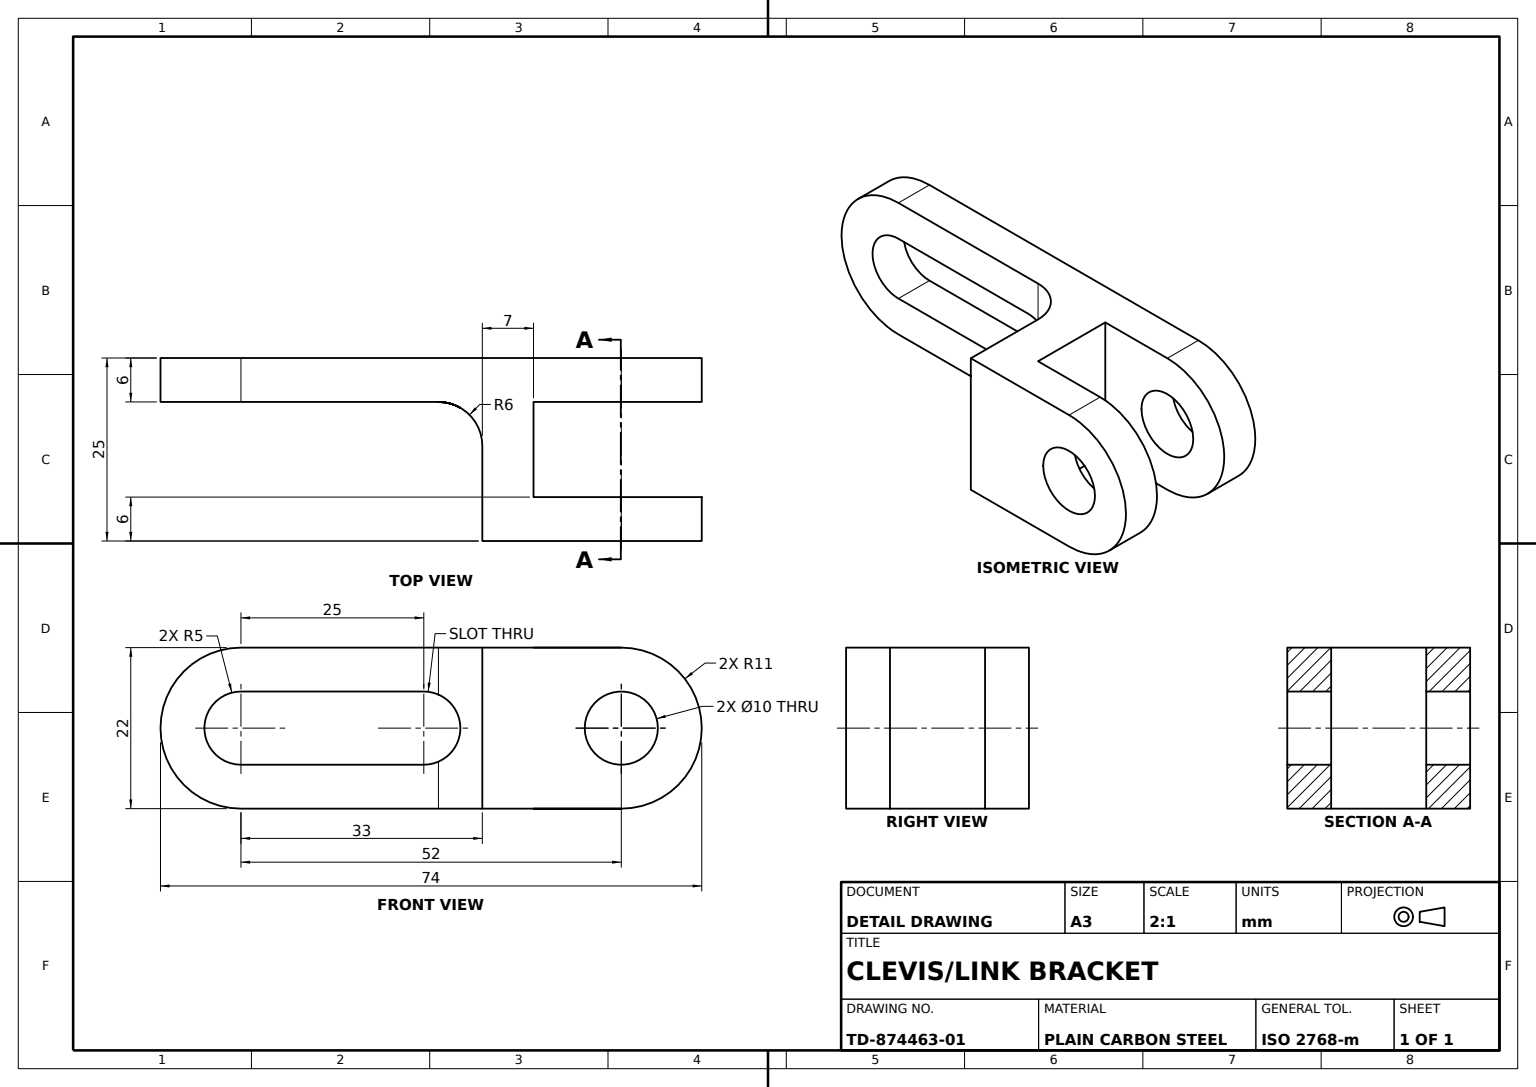
from build123d import *

# Parameters (mm, degrees)
BASE_BLOCK_22X22_DEPTH    = 6
SQUARE_CUTOUT_10X10_DEPTH = 6
LINK_BODY_DEPTH           = 22
LINK_START                = -22
LINK_SLOT_DEPTH           = 22
END_START                 = -6
END_TAB_DEPTH             = 6
CROSS_HOLE_SKETCH_R       = 5
CROSS_HOLE_10_DEPTH       = 25


with BuildPart() as part:
    # Base Block Sketch → Base Block 22x22 (new body)
    with BuildSketch(Plane.XY):
        with BuildLine():
            Line((0, 11), (52, 11))
            ThreePointArc((52, 11), (63, 0), (52, -11))
            Line((52, -11), (0, -11))
            ThreePointArc((0, -11), (-11, 0), (0, 11))
        make_face()
    extrude(amount=BASE_BLOCK_22X22_DEPTH)

    # Square Cutout Sketch → Square Cutout 10x10 (cut)
    with BuildSketch(Plane.XY.offset(6)):
        with BuildLine():
            Line((0, 5), (25, 5))
            ThreePointArc((25, 5), (30, 0), (25, -5))
            Line((25, -5), (0, -5))
            ThreePointArc((0, -5), (-5, 0), (0, 5))
        make_face()
    extrude(amount=-SQUARE_CUTOUT_10X10_DEPTH, mode=Mode.SUBTRACT)

    # Link Profile Sketch → Link Body (add)
    with BuildSketch(Plane.XZ.offset(11)):
        with BuildLine():
            Line((27, 6), (33, 6))
            Line((33, 6), (40, 6))
            Line((40, 6), (40, 19))
            Line((40, 19), (52, 19))
            Line((52, 19), (52, 25))
            Line((52, 25), (33, 25))
            Line((33, 25), (33, 19))
            Line((33, 19), (33, 12))
            ThreePointArc((33, 12), (31.242640687, 7.757359313), (27, 6))
        make_face()
    extrude(amount=-LINK_BODY_DEPTH)

    # Link Slot Sketch → Link Slot (cut)
    with BuildSketch(Plane(origin=(0, 0, 6), x_dir=(-1, 0, 0), z_dir=(0, 0, -1)).offset(LINK_START)):
        with BuildLine():
            Line((-27, 4.582575695), (-27, -4.582575695))
            ThreePointArc((-27, -4.582575695), (-30, 0), (-27, 4.582575695))
        make_face()
    extrude(amount=LINK_SLOT_DEPTH, mode=Mode.SUBTRACT)

    # End Tab Sketch → End Tab (add)
    with BuildSketch(Plane.XY.offset(25).offset(END_START)):
        with BuildLine():
            Line((52, 11), (52, -11))
            ThreePointArc((52, -11), (63, 0), (52, 11))
        make_face()
    extrude(amount=END_TAB_DEPTH)

    # Cross Hole Sketch → Cross Hole Ø10 (cut)
    with BuildSketch(Plane.XY.offset(25)):
        with Locations((52, 0)):
            Circle(CROSS_HOLE_SKETCH_R)
    extrude(amount=-CROSS_HOLE_10_DEPTH, mode=Mode.SUBTRACT)


solid = part.part
